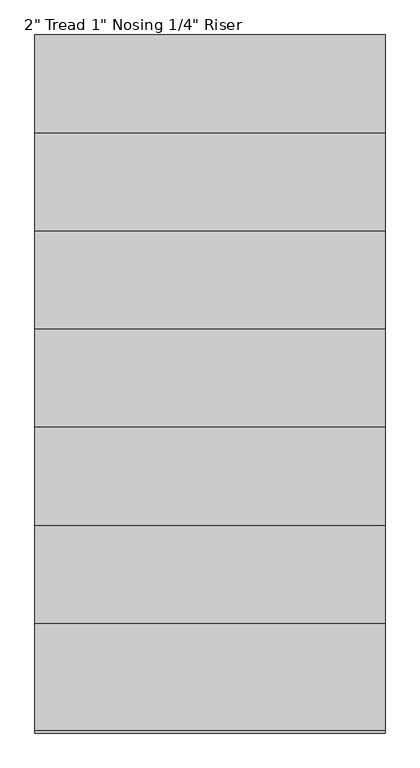
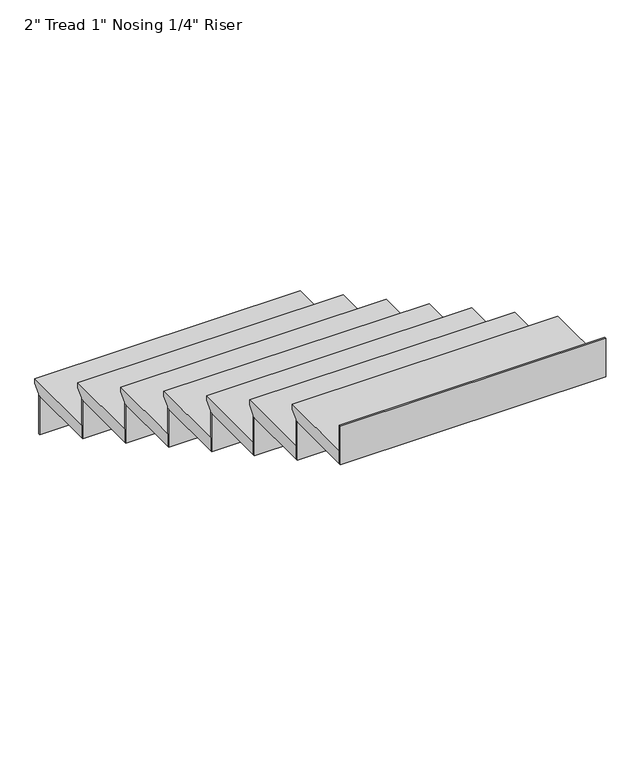
"""IFC4 building model written with IfcOpenShell, lengths in millimetres: stair flight geometry."""

from ifc_helpers import new_model, si_unit, frame, origin, place, context, project, spatial, polyline, outline, extrude, source, transform, mapped, element, save


def stair_flight_d83de971(model_context):
    return source(origin(), model_context, "Body", "SweptSolid", [
        extrude(outline(polyline([(10890.7128362, 2438.4), (11195.5128362, 2438.4), (11195.5128362, 2419.35), (11170.1128362, 2393.95), (11170.1128362, 2387.6), (10890.7128362, 2387.6), (10890.7128362, 2438.4)])), frame((-4958.1002526, 0.0, 0.0), z_axis=(1.0, 0.0, 0.0), x_axis=(0.0, 1.0, 0.0)), (0.0, 0.0, 1.0), 996.95),
        extrude(outline(polyline([(-4958.1002526, 11163.7628362), (-4958.1002526, 11170.1128362), (-3961.1502526, 11170.1128362), (-3961.1502526, 11163.7628362), (-4958.1002526, 11163.7628362)])), frame((0.0, 0.0, 2235.2), z_axis=(0.0, 0.0, 1.0), x_axis=(1.0, 0.0, 0.0)), (0.0, 0.0, 1.0), 152.4),
        extrude(outline(polyline([(-4958.1002526, 10884.3628362), (-4958.1002526, 10890.7128362), (-3961.1502526, 10890.7128362), (-3961.1502526, 10884.3628362), (-4958.1002526, 10884.3628362)])), frame((0.0, 0.0, 2387.6), z_axis=(0.0, 0.0, 1.0), x_axis=(1.0, 0.0, 0.0)), (0.0, 0.0, 1.0), 152.4),
        extrude(outline(polyline([(10611.3128362, 2590.8), (10916.1128362, 2590.8), (10916.1128362, 2571.75), (10890.7128362, 2546.35), (10890.7128362, 2540.0), (10611.3128362, 2540.0), (10611.3128362, 2590.8)])), frame((-4958.1002526, 0.0, 0.0), z_axis=(1.0, 0.0, 0.0), x_axis=(0.0, 1.0, 0.0)), (0.0, 0.0, 1.0), 996.95),
        extrude(outline(polyline([(-4958.1002526, 10604.9628362), (-4958.1002526, 10611.3128362), (-3961.1502526, 10611.3128362), (-3961.1502526, 10604.9628362), (-4958.1002526, 10604.9628362)])), frame((0.0, 0.0, 2540.0), z_axis=(0.0, 0.0, 1.0), x_axis=(1.0, 0.0, 0.0)), (0.0, 0.0, 1.0), 152.4),
        extrude(outline(polyline([(10331.9128362, 2743.2), (10636.7128362, 2743.2), (10636.7128362, 2724.15), (10611.3128362, 2698.75), (10611.3128362, 2692.4), (10331.9128362, 2692.4), (10331.9128362, 2743.2)])), frame((-4958.1002526, 0.0, 0.0), z_axis=(1.0, 0.0, 0.0), x_axis=(0.0, 1.0, 0.0)), (0.0, 0.0, 1.0), 996.95),
        extrude(outline(polyline([(-4958.1002526, 10325.5628362), (-4958.1002526, 10331.9128362), (-3961.1502526, 10331.9128362), (-3961.1502526, 10325.5628362), (-4958.1002526, 10325.5628362)])), frame((0.0, 0.0, 2692.4), z_axis=(0.0, 0.0, 1.0), x_axis=(1.0, 0.0, 0.0)), (0.0, 0.0, 1.0), 152.4),
        extrude(outline(polyline([(10052.5128362, 2895.6), (10357.3128362, 2895.6), (10357.3128362, 2876.55), (10331.9128362, 2851.15), (10331.9128362, 2844.8), (10052.5128362, 2844.8), (10052.5128362, 2895.6)])), frame((-4958.1002526, 0.0, 0.0), z_axis=(1.0, 0.0, 0.0), x_axis=(0.0, 1.0, 0.0)), (0.0, 0.0, 1.0), 996.95),
        extrude(outline(polyline([(-4958.1002526, 10046.1628362), (-4958.1002526, 10052.5128362), (-3961.1502526, 10052.5128362), (-3961.1502526, 10046.1628362), (-4958.1002526, 10046.1628362)])), frame((0.0, 0.0, 2844.8), z_axis=(0.0, 0.0, 1.0), x_axis=(1.0, 0.0, 0.0)), (0.0, 0.0, 1.0), 152.4),
        extrude(outline(polyline([(9773.1128362, 3048.0), (10077.9128362, 3048.0), (10077.9128362, 3028.95), (10052.5128362, 3003.55), (10052.5128362, 2997.2), (9773.1128362, 2997.2), (9773.1128362, 3048.0)])), frame((-4958.1002526, 0.0, 0.0), z_axis=(1.0, 0.0, 0.0), x_axis=(0.0, 1.0, 0.0)), (0.0, 0.0, 1.0), 996.95),
        extrude(outline(polyline([(-4958.1002526, 9766.7628362), (-4958.1002526, 9773.1128362), (-3961.1502526, 9773.1128362), (-3961.1502526, 9766.7628362), (-4958.1002526, 9766.7628362)])), frame((0.0, 0.0, 2997.2), z_axis=(0.0, 0.0, 1.0), x_axis=(1.0, 0.0, 0.0)), (0.0, 0.0, 1.0), 152.4),
        extrude(outline(polyline([(9493.7128362, 3200.4), (9798.5128362, 3200.4), (9798.5128362, 3181.35), (9773.1128362, 3155.95), (9773.1128362, 3149.6), (9493.7128362, 3149.6), (9493.7128362, 3200.4)])), frame((-4958.1002526, 0.0, 0.0), z_axis=(1.0, 0.0, 0.0), x_axis=(0.0, 1.0, 0.0)), (0.0, 0.0, 1.0), 996.95),
        extrude(outline(polyline([(-4958.1002526, 9487.3628362), (-4958.1002526, 9493.7128362), (-3961.1502526, 9493.7128362), (-3961.1502526, 9487.3628362), (-4958.1002526, 9487.3628362)])), frame((0.0, 0.0, 3149.6), z_axis=(0.0, 0.0, 1.0), x_axis=(1.0, 0.0, 0.0)), (0.0, 0.0, 1.0), 152.4),
        extrude(outline(polyline([(-4958.1002526, 9207.9628362), (-4958.1002526, 9214.3128362), (-3961.1502526, 9214.3128362), (-3961.1502526, 9207.9628362), (-4958.1002526, 9207.9628362)])), frame((0.0, 0.0, 3302.0), z_axis=(0.0, 0.0, 1.0), x_axis=(1.0, 0.0, 0.0)), (0.0, 0.0, 1.0), 152.4),
        extrude(outline(polyline([(9214.3128362, 3352.8), (9519.1128362, 3352.8), (9519.1128362, 3333.75), (9493.7128362, 3308.35), (9493.7128362, 3302.0), (9214.3128362, 3302.0), (9214.3128362, 3352.8)])), frame((-4958.1002526, 0.0, 0.0), z_axis=(1.0, 0.0, 0.0), x_axis=(0.0, 1.0, 0.0)), (0.0, 0.0, 1.0), 996.95),
    ])


if __name__ == "__main__":
    model = new_model("IFC4")
    model_context = context("Model", 3, world=origin())
    ifc_project = project(units=[si_unit("LENGTHUNIT", "METRE", prefix="MILLI")], contexts=[model_context])
    site = spatial("IfcSite", under=ifc_project)
    building = spatial("IfcBuilding", under=site)
    placement = place(None, origin())
    stair_flight_shape = stair_flight_d83de971(model_context)
    element("IfcStairFlight", 1, ObjectType="2\" Tread 1\" Nosing 1/4\" Riser", at=placement, inside=building, context=model_context, shape_type="MappedRepresentation", body=[
        mapped(stair_flight_shape, transform((0.0, 0.0, 0.0), x_axis=(1.0, 0.0, 0.0), y_axis=(0.0, 1.0, 0.0), z_axis=(0.0, 0.0, 1.0))),
    ])
    save(model, "model.ifc")
